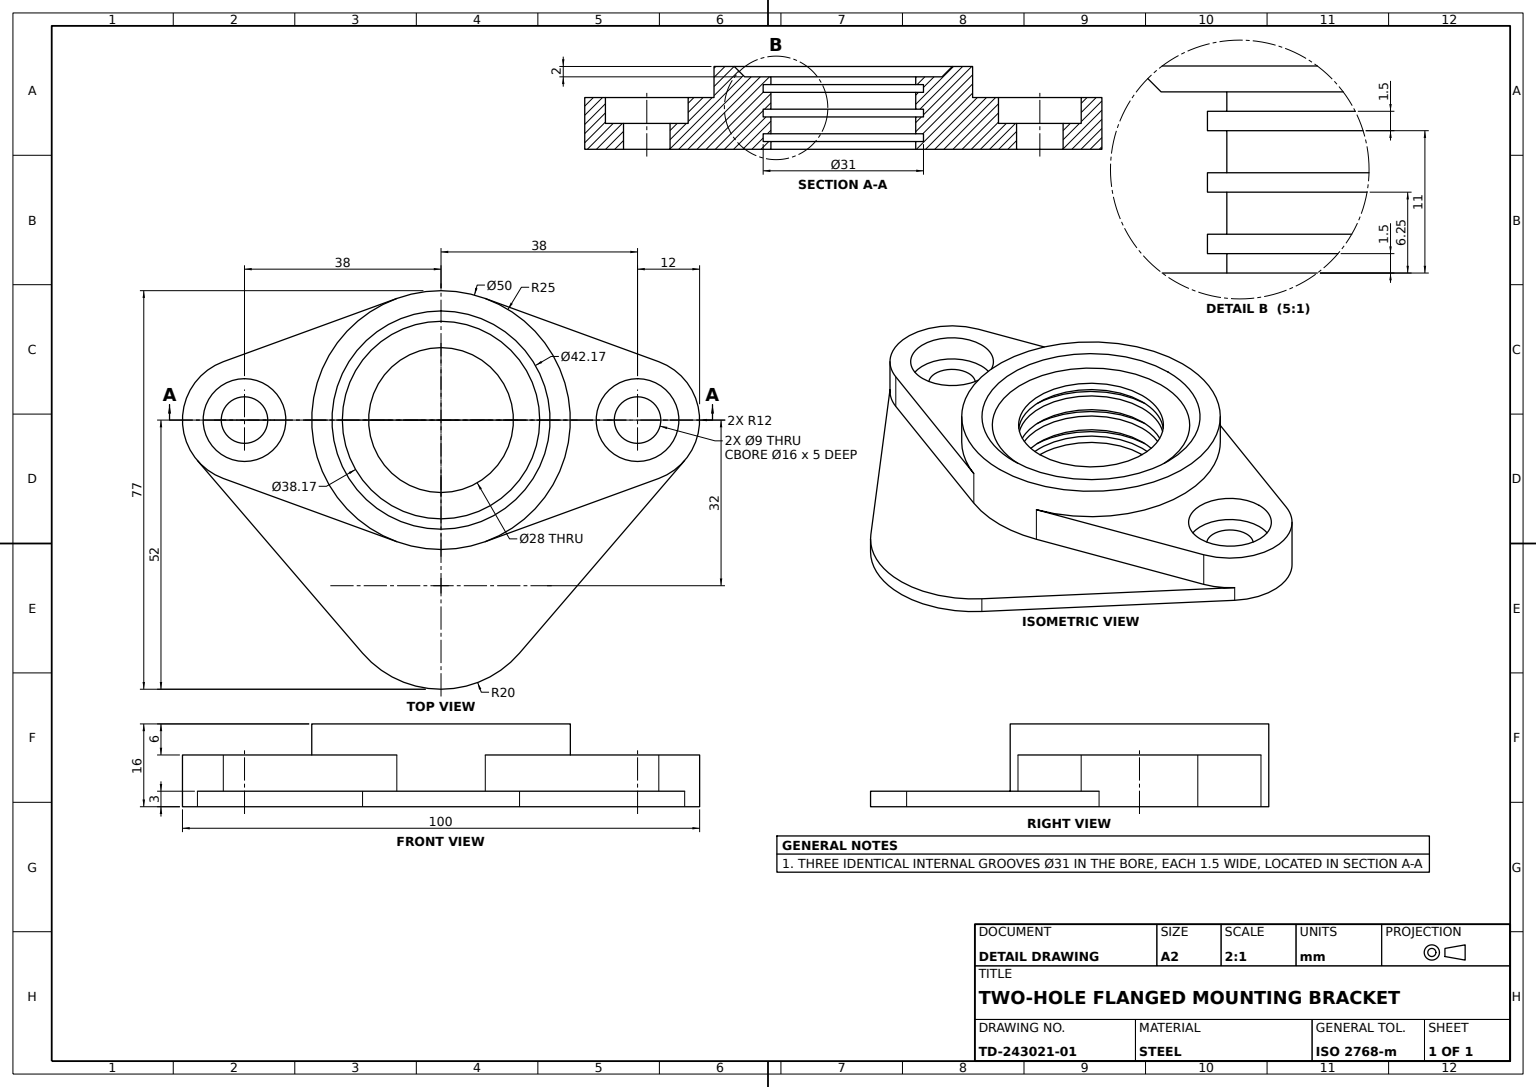
from build123d import *
from build123d.topology import SkipClean

# Parameters (mm, degrees)
BASE_PLATE_DEPTH          = 3
MOUNTING_EARS_DEPTH       = 7
BEARING_HUB_DEPTH         = 13
COUNTERBORE_SKETCH_R      = 8
COUNTERBORES_2X_16_DEPTH  = 5
MOUNTING_HOLE_SKETCH_R    = 4.5
MOUNTING_HOLES_2X_9_DEPTH = 5


with BuildPart() as part:
    # Base Plate Sketch → Base Plate (new body)
    with BuildSketch(Plane(origin=(0, 0, 0), x_dir=(1, 0, 0), z_dir=(0, 1, 0))):
        with BuildLine():
            Line((-42.105263158, 11.275939624), (-8.552631579, 23.491540883))
            ThreePointArc((-8.552631579, 23.491540883), (0, 25), (8.552631579, 23.491540883))
            Line((8.552631579, 23.491540883), (42.105263158, 11.275939624))
            ThreePointArc((42.105263158, 11.275939624), (49.60820541, 3.041310105), (47.10686849, -7.814406331))
            Line((47.10686849, -7.814406331), (15.178114149, -45.024010552))
            ThreePointArc((15.178114149, -45.024010552), (0, -52), (-15.178114149, -45.024010552))
            Line((-15.178114149, -45.024010552), (-47.10686849, -7.814406331))
            ThreePointArc((-47.10686849, -7.814406331), (-49.60820541, 3.041310105), (-42.105263158, 11.275939624))
        make_face()
    extrude(amount=BASE_PLATE_DEPTH)

    # Ear and Hub Profile Sketch → Mounting Ears (add)
    with BuildSketch(Plane(origin=(0, 3, 0), x_dir=(1, 0, 0), z_dir=(0, 1, 0))):
        with BuildLine():
            ThreePointArc((-26, 0), (-31.117527984, -9.830136263), (-42.105263158, -11.275939624))
            Line((-42.105263158, -11.275939624), (-8.552631579, -23.491540883))
            ThreePointArc((-8.552631579, -23.491540883), (-25, 0), (-8.552631579, 23.491540883))
            Line((-8.552631579, 23.491540883), (-42.105263158, 11.275939624))
            ThreePointArc((-42.105263158, 11.275939624), (-31.117527984, 9.830136263), (-26, 0))
        make_face()
        with BuildLine():
            ThreePointArc((-47.10686849, -7.814406331), (-44.829030594, -9.867337085), (-42.105263158, -11.275939624))
            ThreePointArc((-42.105263158, -11.275939624), (-31.117527984, -9.830136263), (-26, 0))
            ThreePointArc((-26, 0), (-31.117527984, 9.830136263), (-42.105263158, 11.275939624))
            ThreePointArc((-42.105263158, 11.275939624), (-49.60820541, 3.041310105), (-47.10686849, -7.814406331))
        make_face()
        with BuildLine():
            ThreePointArc((25, 0), (20.479450548, -14.338483367), (8.552631579, -23.491540883))
            Line((8.552631579, -23.491540883), (42.105263158, -11.275939624))
            ThreePointArc((42.105263158, -11.275939624), (26, 0), (42.105263158, 11.275939624))
            Line((42.105263158, 11.275939624), (8.552631579, 23.491540883))
            ThreePointArc((8.552631579, 23.491540883), (20.479450548, 14.338483367), (25, 0))
        make_face()
        with BuildLine():
            ThreePointArc((42.105263158, 11.275939624), (26, 0), (42.105263158, -11.275939624))
            ThreePointArc((42.105263158, -11.275939624), (44.829030594, -9.867337085), (47.10686849, -7.814406331))
            ThreePointArc((47.10686849, -7.814406331), (49.25349772, -4.166388011), (50, 0))
            ThreePointArc((50, 0), (47.830136263, 6.882472016), (42.105263158, 11.275939624))
        make_face()
    extrude(amount=MOUNTING_EARS_DEPTH)

    # Sketch2_5 → Bearing Hub (add)
    with SkipClean():  # the faces are left unmerged after this step: merging them gives an invalid solid
        with BuildSketch(Plane(origin=(0, 3, 0), x_dir=(1, 0, 0), z_dir=(0, 1, 0))):
            with BuildLine():
                ThreePointArc((-8.552631579, 23.491540883), (-25, 0), (-8.552631579, -23.491540883))
                ThreePointArc((-8.552631579, -23.491540883), (0, -25), (8.552631579, -23.491540883))
                ThreePointArc((8.552631579, -23.491540883), (20.479450548, -14.338483367), (25, 0))
                ThreePointArc((25, 0), (20.479450548, 14.338483367), (8.552631579, 23.491540883))
                ThreePointArc((8.552631579, 23.491540883), (0, 25), (-8.552631579, 23.491540883))
            make_face()
        extrude(amount=BEARING_HUB_DEPTH)

    # Bearing Bore Profile Sketch → Bearing Bore (revolve, cut)
    with SkipClean():  # the faces are left unmerged after this step: merging them gives an invalid solid
        with BuildSketch(Plane.XY, mode=Mode.PRIVATE) as bearing_bore_sk:
            Polygon((21.083967654, 16), (0, 16), (0, 0), (14, 0), (14, 1.5), (15.5, 1.5), (15.5, 3), (14, 3), (14, 6.25), (15.5, 6.25), (15.5, 7.75), (14, 7.75), (14, 11), (15.5, 11), (15.5, 12.5), (14, 12.5), (14, 14), (19.083967654, 14), align=None)
        revolve(bearing_bore_sk.sketch.rotate(Axis((0, 16, 0), (0, -1, 0)), 90), axis=Axis((0, 16, 0), (0, -1, 0)), mode=Mode.SUBTRACT)

    # Counterbore Sketch → Counterbores 2x_16 (cut)
    with SkipClean():  # the faces are left unmerged after this step: merging them gives an invalid solid
        with BuildSketch(Plane(origin=(0, 10, 0), x_dir=(1, 0, 0), z_dir=(0, 1, 0))):
            with Locations(Location((38, 0, 0), (0, 0, 270))):
                Circle(COUNTERBORE_SKETCH_R)
            with Locations(Location((-38, 0, 0), (0, 0, 270))):
                Circle(COUNTERBORE_SKETCH_R)
        extrude(amount=-COUNTERBORES_2X_16_DEPTH, mode=Mode.SUBTRACT)

    # Mounting Hole Sketch → Mounting Holes 2x_9 (cut)
    with SkipClean():  # the faces are left unmerged after this step: merging them gives an invalid solid
        with BuildSketch(Plane(origin=(0, 5, 0), x_dir=(1, 0, 0), z_dir=(0, 1, 0))):
            with Locations(Location((38, 0, 0), (0, 0, 270))):
                Circle(MOUNTING_HOLE_SKETCH_R)
            with Locations(Location((-38, 0, 0), (0, 0, 270))):
                Circle(MOUNTING_HOLE_SKETCH_R)
        extrude(amount=-MOUNTING_HOLES_2X_9_DEPTH, mode=Mode.SUBTRACT)


solid = part.part
